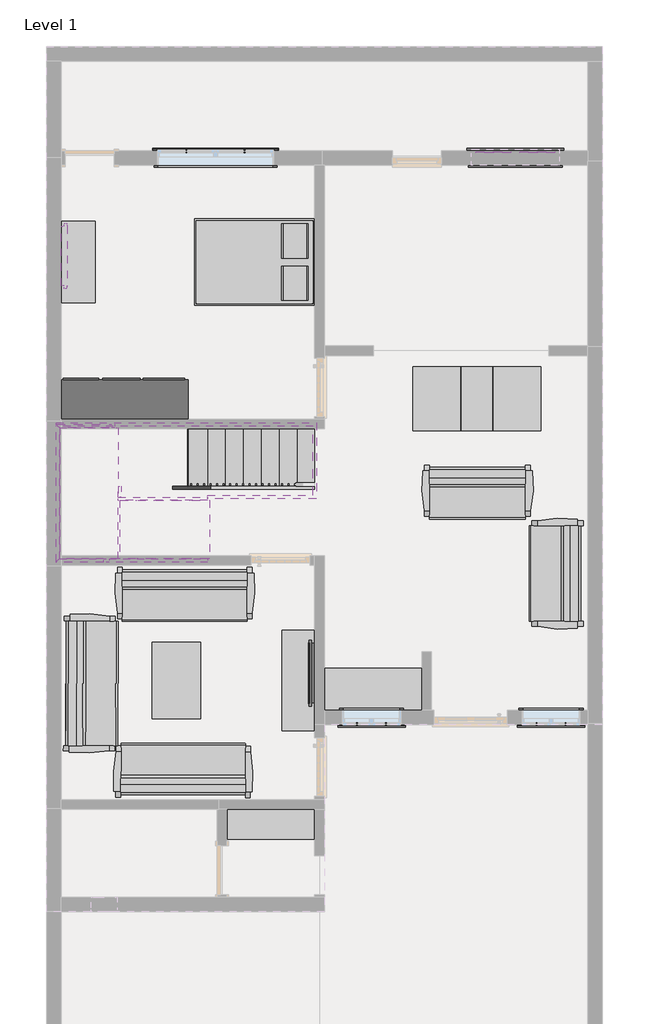
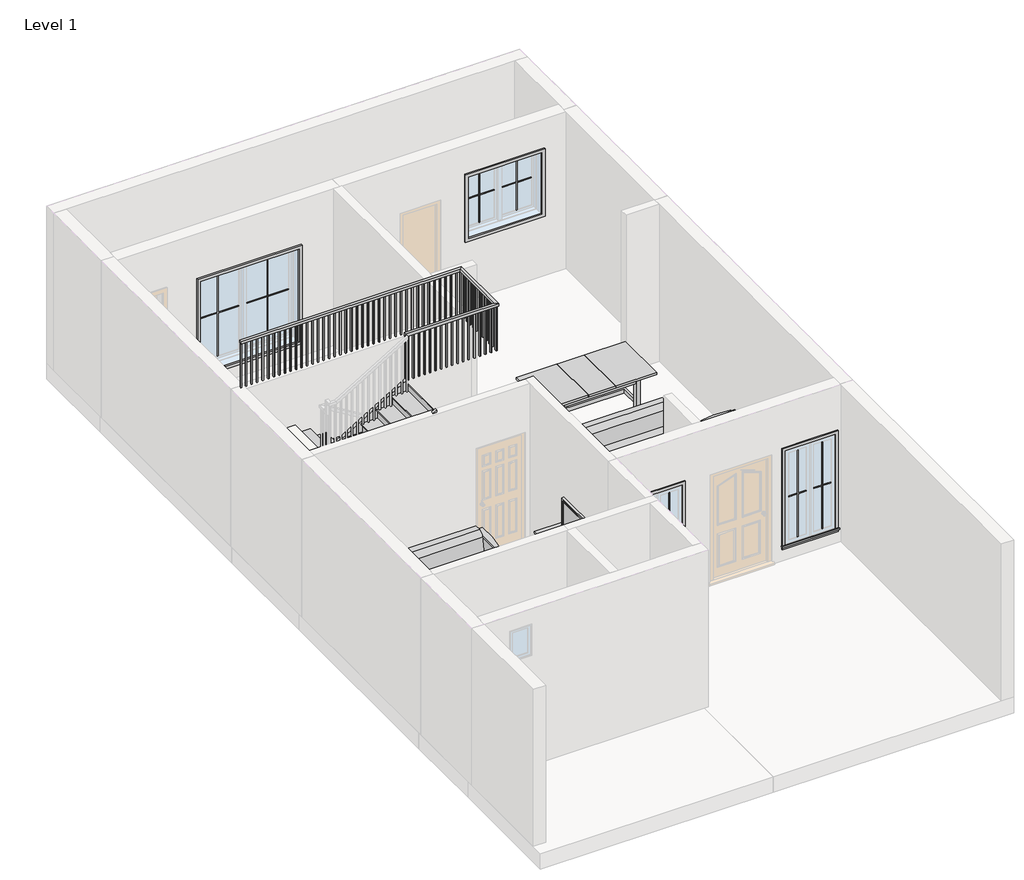
# One storey, part 3 of 3: 19 proxies, 12 furniture elements, 8 members, 2 stair flights, 1 railing, 1 slab.
"""IFC4 building model written with IfcOpenShell, lengths in millimetres."""

from ifc_helpers import new_model, si_unit, frame, origin, place, context, project, spatial, polyline, outline, extrude, faceted_brep, transform, mapped, element, save
from components import generic_models_374839be, muntin_pattern_2x2_muntin_pattern_2x2_0a037076, muntin_pattern_2x2_muntin_pattern_2x2_e6f69628, muntin_pattern_2x2_muntin_pattern_2x2_cdb221ef, muntin_pattern_2x2_muntin_pattern_2x2_811e8f4b, muntin_pattern_2x2_muntin_pattern_2x2_a158773a, muntin_pattern_2x2_muntin_pattern_2x2_9767bead, trim_window_exterior_flat_with_sill_b601e94a, trim_window_exterior_flat_with_sill_5276bcf3, trim_window_exterior_flat_with_sill_c2ca58d6, trim_window_interior_flat_picture_frame_bfefb25c, trim_window_interior_flat_picture_frame_3949a48f, trim_window_interior_flat_picture_frame_d9cdb79e, bath_1_bath_1_5f45cd17, room_1_room_1_fc48c56b, furniture_bed_1_1346x1880x355mm_double_93dec6ea, furniture_sideboard_1220x510x1070mm_0243b4aa, furniture_sideboard_1520x510x970mm_787d3fa7, furniture_sofa_2_1650mm_c7211d0d, furniture_sofa_2_2100x830x380mm_2cdf16e3, furniture_0b97a49d, furniture_table_coffee_glass_1200x760x330mm_bccf866f, furniture_table_dining_w_chairs_rectangular_2000x1000x750mm_b8cbee69, non_monolithic_landing_64c69633, stair_flight_cb879090, stair_flight_6d6c33ab

model = new_model("IFC4")

# Units and contexts
model_context = context("Model", 3, world=origin())
ifc_project = project(units=[si_unit("LENGTHUNIT", "METRE", prefix="MILLI")], contexts=[model_context])

# Site, building, storey
site = spatial("IfcSite", under=ifc_project)
building = spatial("IfcBuilding", under=site)
storey = spatial("IfcBuildingStorey", under=building, Name="Level 1", Elevation=0.0)

# Proxies
placement = place(None, origin())
generic_models_shape = generic_models_374839be(model_context)
element("IfcBuildingElementProxy", 1, Name="Generic Models", at=placement, inside=storey, context=model_context, shape_type="MappedRepresentation", body=[
    mapped(generic_models_shape, transform((0.0, 0.0, 0.0), x_axis=(1.0, 0.0, 0.0), y_axis=(0.0, 1.0, 0.0), z_axis=(0.0, 0.0, 1.0))),
])
muntin_pattern_2x2_muntin_pattern_2x2_shape = muntin_pattern_2x2_muntin_pattern_2x2_0a037076(model_context)
element("IfcBuildingElementProxy", 2, Name="Muntin Pattern_2x2 : Muntin Pattern_2x2", ObjectType="Muntin Pattern_2x2 : Muntin Pattern_2x2", at=placement, inside=storey, context=model_context, shape_type="MappedRepresentation", body=[
    mapped(muntin_pattern_2x2_muntin_pattern_2x2_shape, transform((-3390.5130972, 7136.1620892, 374.65), x_axis=(1.0, 0.0, 0.0), y_axis=(0.0, 1.0, 0.0), z_axis=(0.0, 0.0, 1.0))),
])
muntin_pattern_2x2_muntin_pattern_2x2_2_shape = muntin_pattern_2x2_muntin_pattern_2x2_e6f69628(model_context)
element("IfcBuildingElementProxy", 3, Name="Muntin Pattern_2x2 : Muntin Pattern_2x2", ObjectType="Muntin Pattern_2x2 : Muntin Pattern_2x2", at=placement, inside=storey, context=model_context, shape_type="MappedRepresentation", body=[
    mapped(muntin_pattern_2x2_muntin_pattern_2x2_2_shape, transform((-2479.2880972, 7136.1620892, 374.65), x_axis=(-1.0, 0.0, 0.0), y_axis=(0.0, -1.0, 0.0), z_axis=(0.0, 0.0, 1.0))),
])
muntin_pattern_2x2_muntin_pattern_2x2_3_shape = muntin_pattern_2x2_muntin_pattern_2x2_cdb221ef(model_context)
element("IfcBuildingElementProxy", 4, Name="Muntin Pattern_2x2 : Muntin Pattern_2x2", ObjectType="Muntin Pattern_2x2 : Muntin Pattern_2x2", at=placement, inside=storey, context=model_context, shape_type="MappedRepresentation", body=[
    mapped(muntin_pattern_2x2_muntin_pattern_2x2_3_shape, transform((1410.0869028, 7136.1620892, 1289.05), x_axis=(1.0, 0.0, 0.0), y_axis=(0.0, 1.0, 0.0), z_axis=(0.0, 0.0, 1.0))),
])
muntin_pattern_2x2_muntin_pattern_2x2_4_shape = muntin_pattern_2x2_muntin_pattern_2x2_811e8f4b(model_context)
element("IfcBuildingElementProxy", 5, Name="Muntin Pattern_2x2 : Muntin Pattern_2x2", ObjectType="Muntin Pattern_2x2 : Muntin Pattern_2x2", at=placement, inside=storey, context=model_context, shape_type="MappedRepresentation", body=[
    mapped(muntin_pattern_2x2_muntin_pattern_2x2_4_shape, transform((2092.7119028, 7136.1620892, 1289.05), x_axis=(-1.0, 0.0, 0.0), y_axis=(0.0, -1.0, 0.0), z_axis=(0.0, 0.0, 1.0))),
])
muntin_pattern_2x2_muntin_pattern_2x2_5_shape = muntin_pattern_2x2_muntin_pattern_2x2_a158773a(model_context)
element("IfcBuildingElementProxy", 6, Name="Muntin Pattern_2x2 : Muntin Pattern_2x2", ObjectType="Muntin Pattern_2x2 : Muntin Pattern_2x2", at=placement, inside=storey, context=model_context, shape_type="MappedRepresentation", body=[
    mapped(muntin_pattern_2x2_muntin_pattern_2x2_5_shape, transform((-269.4880972, -1810.9879108, 374.65), x_axis=(-1.0, 0.0, 0.0), y_axis=(0.0, -1.0, 0.0), z_axis=(0.0, 0.0, 1.0))),
])
element("IfcBuildingElementProxy", 7, Name="Muntin Pattern_2x2 : Muntin Pattern_2x2", ObjectType="Muntin Pattern_2x2 : Muntin Pattern_2x2", at=placement, inside=storey, context=model_context, shape_type="MappedRepresentation", body=[
    mapped(muntin_pattern_2x2_muntin_pattern_2x2_5_shape, transform((2537.2119028, -1810.9879108, 374.65), x_axis=(-1.0, 0.0, 0.0), y_axis=(0.0, -1.0, 0.0), z_axis=(0.0, 0.0, 1.0))),
])
muntin_pattern_2x2_muntin_pattern_2x2_6_shape = muntin_pattern_2x2_muntin_pattern_2x2_9767bead(model_context)
element("IfcBuildingElementProxy", 8, Name="Muntin Pattern_2x2 : Muntin Pattern_2x2", ObjectType="Muntin Pattern_2x2 : Muntin Pattern_2x2", at=placement, inside=storey, context=model_context, shape_type="MappedRepresentation", body=[
    mapped(muntin_pattern_2x2_muntin_pattern_2x2_6_shape, transform((-723.5130972, -1810.9879108, 374.65), x_axis=(1.0, 0.0, 0.0), y_axis=(0.0, 1.0, 0.0), z_axis=(0.0, 0.0, 1.0))),
])
element("IfcBuildingElementProxy", 9, Name="Muntin Pattern_2x2 : Muntin Pattern_2x2", ObjectType="Muntin Pattern_2x2 : Muntin Pattern_2x2", at=placement, inside=storey, context=model_context, shape_type="MappedRepresentation", body=[
    mapped(muntin_pattern_2x2_muntin_pattern_2x2_6_shape, transform((2083.1869028, -1810.9879108, 374.65), x_axis=(1.0, 0.0, 0.0), y_axis=(0.0, 1.0, 0.0), z_axis=(0.0, 0.0, 1.0))),
])
trim_window_exterior_flat_with_sill_shape = trim_window_exterior_flat_with_sill_b601e94a(model_context)
element("IfcBuildingElementProxy", 10, Name="Trim-Window-Exterior-Flat : with Sill", ObjectType="Trim-Window-Exterior-Flat : with Sill", at=placement, inside=storey, context=model_context, shape_type="MappedRepresentation", body=[
    mapped(trim_window_exterior_flat_with_sill_shape, transform((-2934.9005972, 7145.6870892, 2133.6), x_axis=(-1.0, 0.0, 0.0), y_axis=(0.0, 0.0, 1.0), z_axis=(0.0, 1.0, 0.0))),
])
trim_window_exterior_flat_with_sill_2_shape = trim_window_exterior_flat_with_sill_5276bcf3(model_context)
element("IfcBuildingElementProxy", 11, Name="Trim-Window-Exterior-Flat : with Sill", ObjectType="Trim-Window-Exterior-Flat : with Sill", at=placement, inside=storey, context=model_context, shape_type="MappedRepresentation", body=[
    mapped(trim_window_exterior_flat_with_sill_2_shape, transform((1751.3994028, 7145.6870892, 2438.4), x_axis=(-1.0, 0.0, 0.0), y_axis=(0.0, 0.0, 1.0), z_axis=(0.0, 1.0, 0.0))),
])
trim_window_exterior_flat_with_sill_3_shape = trim_window_exterior_flat_with_sill_c2ca58d6(model_context)
element("IfcBuildingElementProxy", 12, Name="Trim-Window-Exterior-Flat : with Sill", ObjectType="Trim-Window-Exterior-Flat : with Sill", at=placement, inside=storey, context=model_context, shape_type="MappedRepresentation", body=[
    mapped(trim_window_exterior_flat_with_sill_3_shape, transform((-496.5005972, -1820.5129108, 2133.6), x_axis=(1.0, 0.0, 0.0), y_axis=(0.0, 0.0, 1.0), z_axis=(0.0, -1.0, 0.0))),
])
element("IfcBuildingElementProxy", 13, Name="Trim-Window-Exterior-Flat : with Sill", ObjectType="Trim-Window-Exterior-Flat : with Sill", at=placement, inside=storey, context=model_context, shape_type="MappedRepresentation", body=[
    mapped(trim_window_exterior_flat_with_sill_3_shape, transform((2310.1994028, -1820.5129108, 2133.6), x_axis=(1.0, 0.0, 0.0), y_axis=(0.0, 0.0, 1.0), z_axis=(0.0, -1.0, 0.0))),
])
trim_window_interior_flat_picture_frame_shape = trim_window_interior_flat_picture_frame_bfefb25c(model_context)
element("IfcBuildingElementProxy", 14, Name="Trim-Window-Interior-Flat : Picture Frame", ObjectType="Trim-Window-Interior-Flat : Picture Frame", at=placement, inside=storey, context=model_context, shape_type="MappedRepresentation", body=[
    mapped(trim_window_interior_flat_picture_frame_shape, transform((-2934.9005972, 6917.0870892, 2133.6), x_axis=(1.0, 0.0, 0.0), y_axis=(0.0, 0.0, 1.0), z_axis=(0.0, -1.0, 0.0))),
])
trim_window_interior_flat_picture_frame_2_shape = trim_window_interior_flat_picture_frame_3949a48f(model_context)
element("IfcBuildingElementProxy", 15, Name="Trim-Window-Interior-Flat : Picture Frame", ObjectType="Trim-Window-Interior-Flat : Picture Frame", at=placement, inside=storey, context=model_context, shape_type="MappedRepresentation", body=[
    mapped(trim_window_interior_flat_picture_frame_2_shape, transform((1751.3994028, 6917.0870892, 2438.4), x_axis=(1.0, 0.0, 0.0), y_axis=(0.0, 0.0, 1.0), z_axis=(0.0, -1.0, 0.0))),
])
trim_window_interior_flat_picture_frame_3_shape = trim_window_interior_flat_picture_frame_d9cdb79e(model_context)
element("IfcBuildingElementProxy", 16, Name="Trim-Window-Interior-Flat : Picture Frame", ObjectType="Trim-Window-Interior-Flat : Picture Frame", at=placement, inside=storey, context=model_context, shape_type="MappedRepresentation", body=[
    mapped(trim_window_interior_flat_picture_frame_3_shape, transform((-496.5005972, -1591.9129108, 2133.6), x_axis=(-1.0, 0.0, 0.0), y_axis=(0.0, 0.0, 1.0), z_axis=(0.0, 1.0, 0.0))),
])
element("IfcBuildingElementProxy", 17, Name="Trim-Window-Interior-Flat : Picture Frame", ObjectType="Trim-Window-Interior-Flat : Picture Frame", at=placement, inside=storey, context=model_context, shape_type="MappedRepresentation", body=[
    mapped(trim_window_interior_flat_picture_frame_3_shape, transform((2310.1994028, -1591.9129108, 2133.6), x_axis=(-1.0, 0.0, 0.0), y_axis=(0.0, 0.0, 1.0), z_axis=(0.0, 1.0, 0.0))),
])
bath_1_bath_1_shape = bath_1_bath_1_5f45cd17(model_context)
element("IfcBuildingElementProxy", 18, Name="bath 1 : bath 1", ObjectType="bath 1 : bath 1", at=placement, inside=storey, context=model_context, shape_type="MappedRepresentation", body=[
    mapped(bath_1_bath_1_shape, transform((0.0, 0.0, 0.0), x_axis=(1.0, 0.0, 0.0), y_axis=(0.0, 1.0, 0.0), z_axis=(0.0, 0.0, 1.0))),
])
room_1_room_1_shape = room_1_room_1_fc48c56b(model_context)
element("IfcBuildingElementProxy", 19, Name="room 1 : room 1", ObjectType="room 1 : room 1", at=placement, inside=storey, context=model_context, shape_type="MappedRepresentation", body=[
    mapped(room_1_room_1_shape, transform((0.0, 0.0, 0.0), x_axis=(1.0, 0.0, 0.0), y_axis=(0.0, 1.0, 0.0), z_axis=(0.0, 0.0, 1.0))),
])

# Furniture
furniture_bed_1_1346x1880x355mm_double_shape = furniture_bed_1_1346x1880x355mm_double_93dec6ea(model_context)
element("IfcFurniture", 20, ObjectType="Furniture_Bed_1 : 1346x1880x355mm-Double", at=placement, inside=storey, context=model_context, shape_type="MappedRepresentation", body=[
    mapped(furniture_bed_1_1346x1880x355mm_double_shape, transform((-2091.071089, 5744.8395482, 0.0), x_axis=(0.0, -1.0, 0.0), y_axis=(1.0, 0.0, 0.0), z_axis=(0.0, 0.0, 1.0))),
])
furniture_sideboard_1220x510x1070mm_shape = furniture_sideboard_1220x510x1070mm_0243b4aa(model_context)
element("IfcFurniture", 21, ObjectType="Furniture_Sideboard : 1220x510x1070mm", at=placement, inside=storey, context=model_context, shape_type="MappedRepresentation", body=[
    mapped(furniture_sideboard_1220x510x1070mm_shape, transform((-5458.0635513, 5700.280349, 0.0), x_axis=(0.0, 1.0, 0.0), y_axis=(-1.0, 0.0, 0.0), z_axis=(0.0, 0.0, 1.0))),
])
furniture_sideboard_1520x510x970mm_shape = furniture_sideboard_1520x510x970mm_787d3fa7(model_context)
element("IfcFurniture", 22, ObjectType="Furniture_Sideboard : 1520x510x970mm", at=placement, inside=storey, context=model_context, shape_type="MappedRepresentation", body=[
    mapped(furniture_sideboard_1520x510x970mm_shape, transform((-2003.6635513, -836.9734915, 0.0), x_axis=(0.0, 1.0, 0.0), y_axis=(-1.0, 0.0, 0.0), z_axis=(0.0, 0.0, 1.0))),
])
furniture_sofa_2_1650mm_shape = furniture_sofa_2_1650mm_c7211d0d(model_context)
element("IfcFurniture", 23, ObjectType="Furniture_Sofa_2 : 1650mm", at=placement, inside=storey, context=model_context, shape_type="MappedRepresentation", body=[
    mapped(furniture_sofa_2_1650mm_shape, transform((2109.2895667, 820.2933392, 0.0), x_axis=(0.0, -1.0, 0.0), y_axis=(1.0, 0.0, 0.0), z_axis=(0.0, 0.0, 1.0))),
])
element("IfcFurniture", 24, ObjectType="Furniture_Sofa_2 : 1650mm", at=placement, inside=storey, context=model_context, shape_type="MappedRepresentation", body=[
    mapped(furniture_sofa_2_1650mm_shape, transform((880.1212465, 1534.5772531, 0.0), x_axis=(1.0, 0.0, 0.0), y_axis=(0.0, 1.0, 0.0), z_axis=(0.0, 0.0, 1.0))),
])
furniture_sofa_2_2100x830x380mm_shape = furniture_sofa_2_2100x830x380mm_2cdf16e3(model_context)
element("IfcFurniture", 25, ObjectType="Furniture_Sofa_2 : 2100x830x380mm", at=placement, inside=storey, context=model_context, shape_type="MappedRepresentation", body=[
    mapped(furniture_sofa_2_2100x830x380mm_shape, transform((-4606.7733815, -1454.7297414, 0.0), x_axis=(0.004438895051769032, 0.9999901480568293, 0.0), y_axis=(-0.9999901480568293, 0.004438895051769032, 0.0), z_axis=(0.0, 0.0, 1.0))),
])
element("IfcFurniture", 26, ObjectType="Furniture_Sofa_2 : 2100x830x380mm", at=placement, inside=storey, context=model_context, shape_type="MappedRepresentation", body=[
    mapped(furniture_sofa_2_2100x830x380mm_shape, transform((-3161.0077895, -2253.3666662, 0.0), x_axis=(-0.9999901480568293, 0.004438895051769032, 0.0), y_axis=(-0.004438895051769032, -0.9999901480568293, 0.0), z_axis=(0.0, 0.0, 1.0))),
])
element("IfcFurniture", 27, ObjectType="Furniture_Sofa_2 : 2100x830x380mm", at=placement, inside=storey, context=model_context, shape_type="MappedRepresentation", body=[
    mapped(furniture_sofa_2_2100x830x380mm_shape, transform((-3696.1068472, -65.6227469, 0.0), x_axis=(1.0, 0.0, 0.0), y_axis=(0.0, 1.0, 0.0), z_axis=(0.0, 0.0, 1.0))),
])
furniture_shape = furniture_0b97a49d(model_context)
element("IfcFurniture", 28, ObjectType="Furniture_TV_Plasma : 42\"", at=placement, inside=storey, context=model_context, shape_type="MappedRepresentation", body=[
    mapped(furniture_shape, transform((-1385.5005972, -956.9129108, 914.4), x_axis=(0.0, -1.0, 0.0), y_axis=(1.0, 0.0, 0.0), z_axis=(0.0, 0.0, 1.0))),
])
element("IfcFurniture", 29, ObjectType="Furniture_TV_Plasma : 42\"", at=placement, inside=storey, context=model_context, shape_type="MappedRepresentation", body=[
    mapped(furniture_shape, transform((-5347.9005972, 5444.1870892, 1219.2), x_axis=(0.0, 1.0, 0.0), y_axis=(-1.0, 0.0, 0.0), z_axis=(0.0, 0.0, 1.0))),
])
furniture_table_coffee_glass_1200x760x330mm_shape = furniture_table_coffee_glass_1200x760x330mm_bccf866f(model_context)
element("IfcFurniture", 30, ObjectType="Furniture_Table_Coffee_Glass : 1200x760x330mm", at=placement, inside=storey, context=model_context, shape_type="MappedRepresentation", body=[
    mapped(furniture_table_coffee_glass_1200x760x330mm_shape, transform((-3180.2784522, -1733.8037647, 0.0), x_axis=(0.0, 1.0, 0.0), y_axis=(-1.0, 0.0, 0.0), z_axis=(0.0, 0.0, 1.0))),
])
furniture_table_dining_w_chairs_rectangular_2000x1000x750mm_shape = furniture_table_dining_w_chairs_rectangular_2000x1000x750mm_b8cbee69(model_context)
element("IfcFurniture", 31, ObjectType="Furniture_Table_Dining_w-Chairs_Rectangular : 2000x1000x750mm_w-4_Seats", at=placement, inside=storey, context=model_context, shape_type="MappedRepresentation", body=[
    mapped(furniture_table_dining_w_chairs_rectangular_2000x1000x750mm_shape, transform((1034.1657547, 3225.7786522, 0.0), x_axis=(1.0, 0.0, 0.0), y_axis=(0.0, 1.0, 0.0), z_axis=(0.0, 0.0, 1.0))),
])

# Members
element("IfcMember", 32, ObjectType="Stringer - 2\" Width", at=placement, inside=storey, context=model_context, shape_type="SweptSolid", body=[
    extrude(outline(polyline([(0.0, -1385.5005972), (212.114512, -1385.5005972), (2043.9932998, -4408.1005972), (1687.5845383, -4408.1005972), (0.0, -1623.586109), (0.0, -1385.5005972)])), frame((0.0, 1854.295038, 0.0), z_axis=(0.0, 1.0, 0.0), x_axis=(0.0, 0.0, 1.0)), (0.0, 0.0, 1.0), 50.8),
])
element("IfcMember", 33, ObjectType="Stringer - 2\" Width", at=placement, inside=storey, context=model_context, shape_type="SweptSolid", body=[
    extrude(outline(polyline([(0.0, -1385.5005972), (212.114512, -1385.5005972), (2108.2, -4514.0416525), (1803.4, -4599.196109), (0.0, -1623.586109), (0.0, -1385.5005972)])), frame((0.0, 2819.495038, 0.0), z_axis=(0.0, 1.0, 0.0), x_axis=(0.0, 0.0, 1.0)), (0.0, 0.0, 1.0), 50.8),
])
element("IfcMember", 34, ObjectType="Stringer - 2\" Width", at=placement, inside=storey, context=model_context, shape_type="SweptSolid", body=[
    extrude(outline(polyline([(2244.114512, -4458.9005972), (1887.7057504, -4458.9005972), (2734.3724171, -3061.9005972), (3090.7811786, -3061.9005972), (2244.114512, -4458.9005972)])), frame((0.0, 1684.6870892, 0.0), z_axis=(0.0, 1.0, 0.0), x_axis=(0.0, 0.0, 1.0)), (0.0, 0.0, 1.0), 50.8),
])
element("IfcMember", 35, ObjectType="Stringer - 2\" Width", at=placement, inside=storey, context=model_context, shape_type="SweptSolid", body=[
    extrude(outline(polyline([(2108.2, -4683.1595419), (1803.4, -4598.0050854), (2734.3724171, -3061.9005972), (3090.7811786, -3061.9005972), (2108.2, -4683.1595419)])), frame((0.0, 719.4870892, 0.0), z_axis=(0.0, 1.0, 0.0), x_axis=(0.0, 0.0, 1.0)), (0.0, 0.0, 1.0), 50.8),
])
element("IfcMember", 36, ObjectType="Stringer - 2\" Width", at=placement, inside=storey, context=model_context, shape_type="SweptSolid", body=[
    extrude(outline(polyline([(-4408.1005972, 1735.4870892), (-4458.9005972, 1735.4870892), (-4458.9005972, 1905.095038), (-4408.1005972, 1905.095038), (-4408.1005972, 1735.4870892)])), frame((0.0, 0.0, 1803.4), z_axis=(0.0, 0.0, 1.0), x_axis=(1.0, 0.0, 0.0)), (0.0, 0.0, 1.0), 304.8),
])
element("IfcMember", 37, ObjectType="Stringer - 2\" Width", at=placement, inside=storey, context=model_context, shape_type="Brep", body=[
    faceted_brep([(-4514.0416525, 2819.495038, 2108.2), (-4514.0416525, 2870.295038, 2108.2), (-5424.1005972, 2870.295038, 2108.2), (-5373.3005972, 2819.495038, 2108.2), (-4599.196109, 2819.495038, 1803.4), (-5373.3005972, 2819.495038, 1803.4), (-4599.196109, 2870.295038, 1803.4), (-5424.1005972, 2870.295038, 1803.4)], [[[0, 1, 2, 3]], [[4, 0, 3, 5]], [[6, 4, 5, 7]], [[1, 6, 7, 2]], [[1, 0, 4, 6]], [[2, 7, 5, 3]]]),
])
element("IfcMember", 38, ObjectType="Stringer - 2\" Width", at=placement, inside=storey, context=model_context, shape_type="SweptSolid", body=[
    extrude(outline(polyline([(-5424.1005972, 2870.295038), (-5373.3005972, 2819.495038), (-5373.3005972, 770.2870892), (-5424.1005972, 719.4870892), (-5424.1005972, 2870.295038)])), frame((0.0, 0.0, 1803.4), z_axis=(0.0, 0.0, 1.0), x_axis=(1.0, 0.0, 0.0)), (0.0, 0.0, 1.0), 304.8),
])
element("IfcMember", 39, ObjectType="Stringer - 2\" Width", at=placement, inside=storey, context=model_context, shape_type="Brep", body=[
    faceted_brep([(-5373.3005972, 770.2870892, 2108.2), (-5424.1005972, 719.4870892, 2108.2), (-4683.1595419, 719.4870892, 2108.2), (-4683.1595419, 770.2870892, 2108.2), (-5373.3005972, 770.2870892, 1803.4), (-4598.0050854, 770.2870892, 1803.4), (-5424.1005972, 719.4870892, 1803.4), (-4598.0050854, 719.4870892, 1803.4)], [[[0, 1, 2, 3]], [[4, 0, 3, 5]], [[6, 4, 5, 7]], [[1, 6, 7, 2]], [[1, 0, 4, 6]], [[2, 7, 5, 3]]]),
])

# Railing
element("IfcRailing", 40, ObjectType="Handrail - Rectangular", at=placement, inside=storey, context=model_context, shape_type="SolidModel", body=[
    faceted_brep([(-5424.1005972, 2895.695038, 3962.4), (-5424.1005972, 2895.695038, 3911.6), (-5424.1005972, 2844.895038, 3911.6), (-5424.1005972, 2844.895038, 3962.4), (-1410.9005972, 2844.895038, 3911.6), (-1410.9005972, 2844.895038, 3962.4), (-1360.1005972, 2895.695038, 3962.4), (-1410.9005972, 1760.8870892, 3911.6), (-1410.9005972, 1760.8870892, 3962.4), (-1360.1005972, 1710.0870892, 3962.4), (-3061.9005972, 1710.0870892, 3962.4), (-3061.9005972, 1760.8870892, 3962.4), (-3061.9005972, 1760.8870892, 3911.6), (-3061.9005972, 1710.0870892, 3911.6), (-1360.1005972, 2895.695038, 3911.6), (-1360.1005972, 1710.0870892, 3911.6)], [[[0, 1, 2, 3]], [[3, 2, 4, 5]], [[0, 3, 5, 6]], [[5, 4, 7, 8]], [[6, 5, 8, 9]], [[10, 11, 12, 13]], [[8, 7, 12, 11]], [[9, 8, 11, 10]], [[1, 0, 6, 14]], [[2, 1, 14, 4]], [[14, 6, 9, 15]], [[4, 14, 15, 7]], [[15, 9, 10, 13]], [[7, 15, 13, 12]]]),
    extrude(outline(polyline([(-3001.5755972, 1745.0120892), (-3001.5755972, 1725.9620892), (-3020.6255972, 1725.9620892), (-3020.6255972, 1745.0120892), (-3001.5755972, 1745.0120892)])), frame((0.0, 0.0, 3048.0), z_axis=(0.0, 0.0, 1.0), x_axis=(1.0, 0.0, 0.0)), (0.0, 0.0, 1.0), 863.6),
    extrude(outline(polyline([(-2899.9755972, 1745.0120892), (-2899.9755972, 1725.9620892), (-2919.0255972, 1725.9620892), (-2919.0255972, 1745.0120892), (-2899.9755972, 1745.0120892)])), frame((0.0, 0.0, 3048.0), z_axis=(0.0, 0.0, 1.0), x_axis=(1.0, 0.0, 0.0)), (0.0, 0.0, 1.0), 863.6),
    extrude(outline(polyline([(-2798.3755972, 1745.0120892), (-2798.3755972, 1725.9620892), (-2817.4255972, 1725.9620892), (-2817.4255972, 1745.0120892), (-2798.3755972, 1745.0120892)])), frame((0.0, 0.0, 3048.0), z_axis=(0.0, 0.0, 1.0), x_axis=(1.0, 0.0, 0.0)), (0.0, 0.0, 1.0), 863.6),
    extrude(outline(polyline([(-2696.7755972, 1745.0120892), (-2696.7755972, 1725.9620892), (-2715.8255972, 1725.9620892), (-2715.8255972, 1745.0120892), (-2696.7755972, 1745.0120892)])), frame((0.0, 0.0, 3048.0), z_axis=(0.0, 0.0, 1.0), x_axis=(1.0, 0.0, 0.0)), (0.0, 0.0, 1.0), 863.6),
    extrude(outline(polyline([(-2595.1755972, 1745.0120892), (-2595.1755972, 1725.9620892), (-2614.2255972, 1725.9620892), (-2614.2255972, 1745.0120892), (-2595.1755972, 1745.0120892)])), frame((0.0, 0.0, 3048.0), z_axis=(0.0, 0.0, 1.0), x_axis=(1.0, 0.0, 0.0)), (0.0, 0.0, 1.0), 863.6),
    extrude(outline(polyline([(-2493.5755972, 1745.0120892), (-2493.5755972, 1725.9620892), (-2512.6255972, 1725.9620892), (-2512.6255972, 1745.0120892), (-2493.5755972, 1745.0120892)])), frame((0.0, 0.0, 3048.0), z_axis=(0.0, 0.0, 1.0), x_axis=(1.0, 0.0, 0.0)), (0.0, 0.0, 1.0), 863.6),
    extrude(outline(polyline([(-2391.9755972, 1745.0120892), (-2391.9755972, 1725.9620892), (-2411.0255972, 1725.9620892), (-2411.0255972, 1745.0120892), (-2391.9755972, 1745.0120892)])), frame((0.0, 0.0, 3048.0), z_axis=(0.0, 0.0, 1.0), x_axis=(1.0, 0.0, 0.0)), (0.0, 0.0, 1.0), 863.6),
    extrude(outline(polyline([(-2290.3755972, 1745.0120892), (-2290.3755972, 1725.9620892), (-2309.4255972, 1725.9620892), (-2309.4255972, 1745.0120892), (-2290.3755972, 1745.0120892)])), frame((0.0, 0.0, 3048.0), z_axis=(0.0, 0.0, 1.0), x_axis=(1.0, 0.0, 0.0)), (0.0, 0.0, 1.0), 863.6),
    extrude(outline(polyline([(-2188.7755972, 1745.0120892), (-2188.7755972, 1725.9620892), (-2207.8255972, 1725.9620892), (-2207.8255972, 1745.0120892), (-2188.7755972, 1745.0120892)])), frame((0.0, 0.0, 3048.0), z_axis=(0.0, 0.0, 1.0), x_axis=(1.0, 0.0, 0.0)), (0.0, 0.0, 1.0), 863.6),
    extrude(outline(polyline([(-2087.1755972, 1745.0120892), (-2087.1755972, 1725.9620892), (-2106.2255972, 1725.9620892), (-2106.2255972, 1745.0120892), (-2087.1755972, 1745.0120892)])), frame((0.0, 0.0, 3048.0), z_axis=(0.0, 0.0, 1.0), x_axis=(1.0, 0.0, 0.0)), (0.0, 0.0, 1.0), 863.6),
    extrude(outline(polyline([(-1985.5755972, 1745.0120892), (-1985.5755972, 1725.9620892), (-2004.6255972, 1725.9620892), (-2004.6255972, 1745.0120892), (-1985.5755972, 1745.0120892)])), frame((0.0, 0.0, 3048.0), z_axis=(0.0, 0.0, 1.0), x_axis=(1.0, 0.0, 0.0)), (0.0, 0.0, 1.0), 863.6),
    extrude(outline(polyline([(-1883.9755972, 1745.0120892), (-1883.9755972, 1725.9620892), (-1903.0255972, 1725.9620892), (-1903.0255972, 1745.0120892), (-1883.9755972, 1745.0120892)])), frame((0.0, 0.0, 3048.0), z_axis=(0.0, 0.0, 1.0), x_axis=(1.0, 0.0, 0.0)), (0.0, 0.0, 1.0), 863.6),
    extrude(outline(polyline([(-1782.3755972, 1745.0120892), (-1782.3755972, 1725.9620892), (-1801.4255972, 1725.9620892), (-1801.4255972, 1745.0120892), (-1782.3755972, 1745.0120892)])), frame((0.0, 0.0, 3048.0), z_axis=(0.0, 0.0, 1.0), x_axis=(1.0, 0.0, 0.0)), (0.0, 0.0, 1.0), 863.6),
    extrude(outline(polyline([(-1680.7755972, 1745.0120892), (-1680.7755972, 1725.9620892), (-1699.8255972, 1725.9620892), (-1699.8255972, 1745.0120892), (-1680.7755972, 1745.0120892)])), frame((0.0, 0.0, 3048.0), z_axis=(0.0, 0.0, 1.0), x_axis=(1.0, 0.0, 0.0)), (0.0, 0.0, 1.0), 863.6),
    extrude(outline(polyline([(-1579.1755972, 1745.0120892), (-1579.1755972, 1725.9620892), (-1598.2255972, 1725.9620892), (-1598.2255972, 1745.0120892), (-1579.1755972, 1745.0120892)])), frame((0.0, 0.0, 3048.0), z_axis=(0.0, 0.0, 1.0), x_axis=(1.0, 0.0, 0.0)), (0.0, 0.0, 1.0), 863.6),
    extrude(outline(polyline([(-1477.5755972, 1745.0120892), (-1477.5755972, 1725.9620892), (-1496.6255972, 1725.9620892), (-1496.6255972, 1745.0120892), (-1477.5755972, 1745.0120892)])), frame((0.0, 0.0, 3048.0), z_axis=(0.0, 0.0, 1.0), x_axis=(1.0, 0.0, 0.0)), (0.0, 0.0, 1.0), 863.6),
    extrude(outline(polyline([(-1395.0255972, 1762.220038), (-1375.9755972, 1762.220038), (-1375.9755972, 1743.170038), (-1395.0255972, 1743.170038), (-1395.0255972, 1762.220038)])), frame((0.0, 0.0, 3048.0), z_axis=(0.0, 0.0, 1.0), x_axis=(1.0, 0.0, 0.0)), (0.0, 0.0, 1.0), 863.6),
    extrude(outline(polyline([(-1395.0255972, 1863.820038), (-1375.9755972, 1863.820038), (-1375.9755972, 1844.770038), (-1395.0255972, 1844.770038), (-1395.0255972, 1863.820038)])), frame((0.0, 0.0, 3048.0), z_axis=(0.0, 0.0, 1.0), x_axis=(1.0, 0.0, 0.0)), (0.0, 0.0, 1.0), 863.6),
    extrude(outline(polyline([(-1395.0255972, 1965.420038), (-1375.9755972, 1965.420038), (-1375.9755972, 1946.370038), (-1395.0255972, 1946.370038), (-1395.0255972, 1965.420038)])), frame((0.0, 0.0, 3048.0), z_axis=(0.0, 0.0, 1.0), x_axis=(1.0, 0.0, 0.0)), (0.0, 0.0, 1.0), 863.6),
    extrude(outline(polyline([(-1395.0255972, 2067.020038), (-1375.9755972, 2067.020038), (-1375.9755972, 2047.970038), (-1395.0255972, 2047.970038), (-1395.0255972, 2067.020038)])), frame((0.0, 0.0, 3048.0), z_axis=(0.0, 0.0, 1.0), x_axis=(1.0, 0.0, 0.0)), (0.0, 0.0, 1.0), 863.6),
    extrude(outline(polyline([(-1395.0255972, 2168.620038), (-1375.9755972, 2168.620038), (-1375.9755972, 2149.570038), (-1395.0255972, 2149.570038), (-1395.0255972, 2168.620038)])), frame((0.0, 0.0, 3048.0), z_axis=(0.0, 0.0, 1.0), x_axis=(1.0, 0.0, 0.0)), (0.0, 0.0, 1.0), 863.6),
    extrude(outline(polyline([(-1395.0255972, 2270.220038), (-1375.9755972, 2270.220038), (-1375.9755972, 2251.170038), (-1395.0255972, 2251.170038), (-1395.0255972, 2270.220038)])), frame((0.0, 0.0, 3048.0), z_axis=(0.0, 0.0, 1.0), x_axis=(1.0, 0.0, 0.0)), (0.0, 0.0, 1.0), 863.6),
    extrude(outline(polyline([(-1395.0255972, 2371.820038), (-1375.9755972, 2371.820038), (-1375.9755972, 2352.770038), (-1395.0255972, 2352.770038), (-1395.0255972, 2371.820038)])), frame((0.0, 0.0, 3048.0), z_axis=(0.0, 0.0, 1.0), x_axis=(1.0, 0.0, 0.0)), (0.0, 0.0, 1.0), 863.6),
    extrude(outline(polyline([(-1395.0255972, 2473.420038), (-1375.9755972, 2473.420038), (-1375.9755972, 2454.370038), (-1395.0255972, 2454.370038), (-1395.0255972, 2473.420038)])), frame((0.0, 0.0, 3048.0), z_axis=(0.0, 0.0, 1.0), x_axis=(1.0, 0.0, 0.0)), (0.0, 0.0, 1.0), 863.6),
    extrude(outline(polyline([(-1395.0255972, 2575.020038), (-1375.9755972, 2575.020038), (-1375.9755972, 2555.970038), (-1395.0255972, 2555.970038), (-1395.0255972, 2575.020038)])), frame((0.0, 0.0, 3048.0), z_axis=(0.0, 0.0, 1.0), x_axis=(1.0, 0.0, 0.0)), (0.0, 0.0, 1.0), 863.6),
    extrude(outline(polyline([(-1395.0255972, 2676.620038), (-1375.9755972, 2676.620038), (-1375.9755972, 2657.570038), (-1395.0255972, 2657.570038), (-1395.0255972, 2676.620038)])), frame((0.0, 0.0, 3048.0), z_axis=(0.0, 0.0, 1.0), x_axis=(1.0, 0.0, 0.0)), (0.0, 0.0, 1.0), 863.6),
    extrude(outline(polyline([(-1395.0255972, 2778.220038), (-1375.9755972, 2778.220038), (-1375.9755972, 2759.170038), (-1395.0255972, 2759.170038), (-1395.0255972, 2778.220038)])), frame((0.0, 0.0, 3048.0), z_axis=(0.0, 0.0, 1.0), x_axis=(1.0, 0.0, 0.0)), (0.0, 0.0, 1.0), 863.6),
    extrude(outline(polyline([(-1471.2255972, 2860.770038), (-1471.2255972, 2879.820038), (-1452.1755972, 2879.820038), (-1452.1755972, 2860.770038), (-1471.2255972, 2860.770038)])), frame((0.0, 0.0, 3048.0), z_axis=(0.0, 0.0, 1.0), x_axis=(1.0, 0.0, 0.0)), (0.0, 0.0, 1.0), 863.6),
    extrude(outline(polyline([(-1572.8255972, 2860.770038), (-1572.8255972, 2879.820038), (-1553.7755972, 2879.820038), (-1553.7755972, 2860.770038), (-1572.8255972, 2860.770038)])), frame((0.0, 0.0, 3048.0), z_axis=(0.0, 0.0, 1.0), x_axis=(1.0, 0.0, 0.0)), (0.0, 0.0, 1.0), 863.6),
    extrude(outline(polyline([(-1674.4255972, 2860.770038), (-1674.4255972, 2879.820038), (-1655.3755972, 2879.820038), (-1655.3755972, 2860.770038), (-1674.4255972, 2860.770038)])), frame((0.0, 0.0, 3048.0), z_axis=(0.0, 0.0, 1.0), x_axis=(1.0, 0.0, 0.0)), (0.0, 0.0, 1.0), 863.6),
    extrude(outline(polyline([(-1776.0255972, 2860.770038), (-1776.0255972, 2879.820038), (-1756.9755972, 2879.820038), (-1756.9755972, 2860.770038), (-1776.0255972, 2860.770038)])), frame((0.0, 0.0, 3048.0), z_axis=(0.0, 0.0, 1.0), x_axis=(1.0, 0.0, 0.0)), (0.0, 0.0, 1.0), 863.6),
    extrude(outline(polyline([(-1877.6255972, 2860.770038), (-1877.6255972, 2879.820038), (-1858.5755972, 2879.820038), (-1858.5755972, 2860.770038), (-1877.6255972, 2860.770038)])), frame((0.0, 0.0, 3048.0), z_axis=(0.0, 0.0, 1.0), x_axis=(1.0, 0.0, 0.0)), (0.0, 0.0, 1.0), 863.6),
    extrude(outline(polyline([(-1979.2255972, 2860.770038), (-1979.2255972, 2879.820038), (-1960.1755972, 2879.820038), (-1960.1755972, 2860.770038), (-1979.2255972, 2860.770038)])), frame((0.0, 0.0, 3048.0), z_axis=(0.0, 0.0, 1.0), x_axis=(1.0, 0.0, 0.0)), (0.0, 0.0, 1.0), 863.6),
    extrude(outline(polyline([(-2080.8255972, 2860.770038), (-2080.8255972, 2879.820038), (-2061.7755972, 2879.820038), (-2061.7755972, 2860.770038), (-2080.8255972, 2860.770038)])), frame((0.0, 0.0, 3048.0), z_axis=(0.0, 0.0, 1.0), x_axis=(1.0, 0.0, 0.0)), (0.0, 0.0, 1.0), 863.6),
    extrude(outline(polyline([(-2182.4255972, 2860.770038), (-2182.4255972, 2879.820038), (-2163.3755972, 2879.820038), (-2163.3755972, 2860.770038), (-2182.4255972, 2860.770038)])), frame((0.0, 0.0, 3048.0), z_axis=(0.0, 0.0, 1.0), x_axis=(1.0, 0.0, 0.0)), (0.0, 0.0, 1.0), 863.6),
    extrude(outline(polyline([(-2284.0255972, 2860.770038), (-2284.0255972, 2879.820038), (-2264.9755972, 2879.820038), (-2264.9755972, 2860.770038), (-2284.0255972, 2860.770038)])), frame((0.0, 0.0, 3048.0), z_axis=(0.0, 0.0, 1.0), x_axis=(1.0, 0.0, 0.0)), (0.0, 0.0, 1.0), 863.6),
    extrude(outline(polyline([(-2385.6255972, 2860.770038), (-2385.6255972, 2879.820038), (-2366.5755972, 2879.820038), (-2366.5755972, 2860.770038), (-2385.6255972, 2860.770038)])), frame((0.0, 0.0, 3048.0), z_axis=(0.0, 0.0, 1.0), x_axis=(1.0, 0.0, 0.0)), (0.0, 0.0, 1.0), 863.6),
    extrude(outline(polyline([(-2487.2255972, 2860.770038), (-2487.2255972, 2879.820038), (-2468.1755972, 2879.820038), (-2468.1755972, 2860.770038), (-2487.2255972, 2860.770038)])), frame((0.0, 0.0, 3048.0), z_axis=(0.0, 0.0, 1.0), x_axis=(1.0, 0.0, 0.0)), (0.0, 0.0, 1.0), 863.6),
    extrude(outline(polyline([(-2588.8255972, 2860.770038), (-2588.8255972, 2879.820038), (-2569.7755972, 2879.820038), (-2569.7755972, 2860.770038), (-2588.8255972, 2860.770038)])), frame((0.0, 0.0, 3048.0), z_axis=(0.0, 0.0, 1.0), x_axis=(1.0, 0.0, 0.0)), (0.0, 0.0, 1.0), 863.6),
    extrude(outline(polyline([(-2690.4255972, 2860.770038), (-2690.4255972, 2879.820038), (-2671.3755972, 2879.820038), (-2671.3755972, 2860.770038), (-2690.4255972, 2860.770038)])), frame((0.0, 0.0, 3048.0), z_axis=(0.0, 0.0, 1.0), x_axis=(1.0, 0.0, 0.0)), (0.0, 0.0, 1.0), 863.6),
    extrude(outline(polyline([(-2792.0255972, 2860.770038), (-2792.0255972, 2879.820038), (-2772.9755972, 2879.820038), (-2772.9755972, 2860.770038), (-2792.0255972, 2860.770038)])), frame((0.0, 0.0, 3048.0), z_axis=(0.0, 0.0, 1.0), x_axis=(1.0, 0.0, 0.0)), (0.0, 0.0, 1.0), 863.6),
    extrude(outline(polyline([(-2893.6255972, 2860.770038), (-2893.6255972, 2879.820038), (-2874.5755972, 2879.820038), (-2874.5755972, 2860.770038), (-2893.6255972, 2860.770038)])), frame((0.0, 0.0, 3048.0), z_axis=(0.0, 0.0, 1.0), x_axis=(1.0, 0.0, 0.0)), (0.0, 0.0, 1.0), 863.6),
    extrude(outline(polyline([(-2995.2255972, 2860.770038), (-2995.2255972, 2879.820038), (-2976.1755972, 2879.820038), (-2976.1755972, 2860.770038), (-2995.2255972, 2860.770038)])), frame((0.0, 0.0, 3048.0), z_axis=(0.0, 0.0, 1.0), x_axis=(1.0, 0.0, 0.0)), (0.0, 0.0, 1.0), 863.6),
    extrude(outline(polyline([(-3096.8255972, 2860.770038), (-3096.8255972, 2879.820038), (-3077.7755972, 2879.820038), (-3077.7755972, 2860.770038), (-3096.8255972, 2860.770038)])), frame((0.0, 0.0, 3048.0), z_axis=(0.0, 0.0, 1.0), x_axis=(1.0, 0.0, 0.0)), (0.0, 0.0, 1.0), 863.6),
    extrude(outline(polyline([(-3198.4255972, 2860.770038), (-3198.4255972, 2879.820038), (-3179.3755972, 2879.820038), (-3179.3755972, 2860.770038), (-3198.4255972, 2860.770038)])), frame((0.0, 0.0, 3048.0), z_axis=(0.0, 0.0, 1.0), x_axis=(1.0, 0.0, 0.0)), (0.0, 0.0, 1.0), 863.6),
    extrude(outline(polyline([(-3300.0255972, 2860.770038), (-3300.0255972, 2879.820038), (-3280.9755972, 2879.820038), (-3280.9755972, 2860.770038), (-3300.0255972, 2860.770038)])), frame((0.0, 0.0, 3048.0), z_axis=(0.0, 0.0, 1.0), x_axis=(1.0, 0.0, 0.0)), (0.0, 0.0, 1.0), 863.6),
    extrude(outline(polyline([(-3401.6255972, 2860.770038), (-3401.6255972, 2879.820038), (-3382.5755972, 2879.820038), (-3382.5755972, 2860.770038), (-3401.6255972, 2860.770038)])), frame((0.0, 0.0, 3048.0), z_axis=(0.0, 0.0, 1.0), x_axis=(1.0, 0.0, 0.0)), (0.0, 0.0, 1.0), 863.6),
    extrude(outline(polyline([(-3503.2255972, 2860.770038), (-3503.2255972, 2879.820038), (-3484.1755972, 2879.820038), (-3484.1755972, 2860.770038), (-3503.2255972, 2860.770038)])), frame((0.0, 0.0, 3048.0), z_axis=(0.0, 0.0, 1.0), x_axis=(1.0, 0.0, 0.0)), (0.0, 0.0, 1.0), 863.6),
    extrude(outline(polyline([(-3604.8255972, 2860.770038), (-3604.8255972, 2879.820038), (-3585.7755972, 2879.820038), (-3585.7755972, 2860.770038), (-3604.8255972, 2860.770038)])), frame((0.0, 0.0, 3048.0), z_axis=(0.0, 0.0, 1.0), x_axis=(1.0, 0.0, 0.0)), (0.0, 0.0, 1.0), 863.6),
    extrude(outline(polyline([(-3706.4255972, 2860.770038), (-3706.4255972, 2879.820038), (-3687.3755972, 2879.820038), (-3687.3755972, 2860.770038), (-3706.4255972, 2860.770038)])), frame((0.0, 0.0, 3048.0), z_axis=(0.0, 0.0, 1.0), x_axis=(1.0, 0.0, 0.0)), (0.0, 0.0, 1.0), 863.6),
    extrude(outline(polyline([(-3808.0255972, 2860.770038), (-3808.0255972, 2879.820038), (-3788.9755972, 2879.820038), (-3788.9755972, 2860.770038), (-3808.0255972, 2860.770038)])), frame((0.0, 0.0, 3048.0), z_axis=(0.0, 0.0, 1.0), x_axis=(1.0, 0.0, 0.0)), (0.0, 0.0, 1.0), 863.6),
    extrude(outline(polyline([(-3909.6255972, 2860.770038), (-3909.6255972, 2879.820038), (-3890.5755972, 2879.820038), (-3890.5755972, 2860.770038), (-3909.6255972, 2860.770038)])), frame((0.0, 0.0, 3048.0), z_axis=(0.0, 0.0, 1.0), x_axis=(1.0, 0.0, 0.0)), (0.0, 0.0, 1.0), 863.6),
    extrude(outline(polyline([(-4011.2255972, 2860.770038), (-4011.2255972, 2879.820038), (-3992.1755972, 2879.820038), (-3992.1755972, 2860.770038), (-4011.2255972, 2860.770038)])), frame((0.0, 0.0, 3048.0), z_axis=(0.0, 0.0, 1.0), x_axis=(1.0, 0.0, 0.0)), (0.0, 0.0, 1.0), 863.6),
    extrude(outline(polyline([(-4112.8255972, 2860.770038), (-4112.8255972, 2879.820038), (-4093.7755972, 2879.820038), (-4093.7755972, 2860.770038), (-4112.8255972, 2860.770038)])), frame((0.0, 0.0, 3048.0), z_axis=(0.0, 0.0, 1.0), x_axis=(1.0, 0.0, 0.0)), (0.0, 0.0, 1.0), 863.6),
    extrude(outline(polyline([(-4214.4255972, 2860.770038), (-4214.4255972, 2879.820038), (-4195.3755972, 2879.820038), (-4195.3755972, 2860.770038), (-4214.4255972, 2860.770038)])), frame((0.0, 0.0, 3048.0), z_axis=(0.0, 0.0, 1.0), x_axis=(1.0, 0.0, 0.0)), (0.0, 0.0, 1.0), 863.6),
    extrude(outline(polyline([(-4316.0255972, 2860.770038), (-4316.0255972, 2879.820038), (-4296.9755972, 2879.820038), (-4296.9755972, 2860.770038), (-4316.0255972, 2860.770038)])), frame((0.0, 0.0, 3048.0), z_axis=(0.0, 0.0, 1.0), x_axis=(1.0, 0.0, 0.0)), (0.0, 0.0, 1.0), 863.6),
    extrude(outline(polyline([(-4417.6255972, 2860.770038), (-4417.6255972, 2879.820038), (-4398.5755972, 2879.820038), (-4398.5755972, 2860.770038), (-4417.6255972, 2860.770038)])), frame((0.0, 0.0, 3048.0), z_axis=(0.0, 0.0, 1.0), x_axis=(1.0, 0.0, 0.0)), (0.0, 0.0, 1.0), 863.6),
    extrude(outline(polyline([(-4519.2255972, 2860.770038), (-4519.2255972, 2879.820038), (-4500.1755972, 2879.820038), (-4500.1755972, 2860.770038), (-4519.2255972, 2860.770038)])), frame((0.0, 0.0, 3048.0), z_axis=(0.0, 0.0, 1.0), x_axis=(1.0, 0.0, 0.0)), (0.0, 0.0, 1.0), 863.6),
    extrude(outline(polyline([(-4620.8255972, 2860.770038), (-4620.8255972, 2879.820038), (-4601.7755972, 2879.820038), (-4601.7755972, 2860.770038), (-4620.8255972, 2860.770038)])), frame((0.0, 0.0, 3048.0), z_axis=(0.0, 0.0, 1.0), x_axis=(1.0, 0.0, 0.0)), (0.0, 0.0, 1.0), 863.6),
    extrude(outline(polyline([(-4722.4255972, 2860.770038), (-4722.4255972, 2879.820038), (-4703.3755972, 2879.820038), (-4703.3755972, 2860.770038), (-4722.4255972, 2860.770038)])), frame((0.0, 0.0, 3048.0), z_axis=(0.0, 0.0, 1.0), x_axis=(1.0, 0.0, 0.0)), (0.0, 0.0, 1.0), 863.6),
    extrude(outline(polyline([(-4824.0255972, 2860.770038), (-4824.0255972, 2879.820038), (-4804.9755972, 2879.820038), (-4804.9755972, 2860.770038), (-4824.0255972, 2860.770038)])), frame((0.0, 0.0, 3048.0), z_axis=(0.0, 0.0, 1.0), x_axis=(1.0, 0.0, 0.0)), (0.0, 0.0, 1.0), 863.6),
    extrude(outline(polyline([(-4925.6255972, 2860.770038), (-4925.6255972, 2879.820038), (-4906.5755972, 2879.820038), (-4906.5755972, 2860.770038), (-4925.6255972, 2860.770038)])), frame((0.0, 0.0, 3048.0), z_axis=(0.0, 0.0, 1.0), x_axis=(1.0, 0.0, 0.0)), (0.0, 0.0, 1.0), 863.6),
    extrude(outline(polyline([(-5027.2255972, 2860.770038), (-5027.2255972, 2879.820038), (-5008.1755972, 2879.820038), (-5008.1755972, 2860.770038), (-5027.2255972, 2860.770038)])), frame((0.0, 0.0, 3048.0), z_axis=(0.0, 0.0, 1.0), x_axis=(1.0, 0.0, 0.0)), (0.0, 0.0, 1.0), 863.6),
    extrude(outline(polyline([(-5128.8255972, 2860.770038), (-5128.8255972, 2879.820038), (-5109.7755972, 2879.820038), (-5109.7755972, 2860.770038), (-5128.8255972, 2860.770038)])), frame((0.0, 0.0, 3048.0), z_axis=(0.0, 0.0, 1.0), x_axis=(1.0, 0.0, 0.0)), (0.0, 0.0, 1.0), 863.6),
    extrude(outline(polyline([(-5230.4255972, 2860.770038), (-5230.4255972, 2879.820038), (-5211.3755972, 2879.820038), (-5211.3755972, 2860.770038), (-5230.4255972, 2860.770038)])), frame((0.0, 0.0, 3048.0), z_axis=(0.0, 0.0, 1.0), x_axis=(1.0, 0.0, 0.0)), (0.0, 0.0, 1.0), 863.6),
    extrude(outline(polyline([(-5332.0255972, 2860.770038), (-5332.0255972, 2879.820038), (-5312.9755972, 2879.820038), (-5312.9755972, 2860.770038), (-5332.0255972, 2860.770038)])), frame((0.0, 0.0, 3048.0), z_axis=(0.0, 0.0, 1.0), x_axis=(1.0, 0.0, 0.0)), (0.0, 0.0, 1.0), 863.6),
    extrude(outline(polyline([(-1395.0255972, 1745.0120892), (-1375.9755972, 1745.0120892), (-1375.9755972, 1725.9620892), (-1395.0255972, 1725.9620892), (-1395.0255972, 1745.0120892)])), frame((0.0, 0.0, 3048.0), z_axis=(0.0, 0.0, 1.0), x_axis=(1.0, 0.0, 0.0)), (0.0, 0.0, 1.0), 863.6),
    extrude(outline(polyline([(-1395.0255972, 2860.770038), (-1395.0255972, 2879.820038), (-1375.9755972, 2879.820038), (-1375.9755972, 2860.770038), (-1395.0255972, 2860.770038)])), frame((0.0, 0.0, 3048.0), z_axis=(0.0, 0.0, 1.0), x_axis=(1.0, 0.0, 0.0)), (0.0, 0.0, 1.0), 863.6),
    extrude(outline(polyline([(-3042.8505972, 1745.0120892), (-3042.8505972, 1725.9620892), (-3061.9005972, 1725.9620892), (-3061.9005972, 1745.0120892), (-3042.8505972, 1745.0120892)])), frame((0.0, 0.0, 3048.0), z_axis=(0.0, 0.0, 1.0), x_axis=(1.0, 0.0, 0.0)), (0.0, 0.0, 1.0), 863.6),
    extrude(outline(polyline([(-5424.1005972, 2860.770038), (-5424.1005972, 2879.820038), (-5405.0505972, 2879.820038), (-5405.0505972, 2860.770038), (-5424.1005972, 2860.770038)])), frame((0.0, 0.0, 3048.0), z_axis=(0.0, 0.0, 1.0), x_axis=(1.0, 0.0, 0.0)), (0.0, 0.0, 1.0), 863.6),
])

# Slab
non_monolithic_landing_shape = non_monolithic_landing_64c69633(model_context)
element("IfcSlab", 41, ObjectType="Non-Monolithic Landing", at=placement, inside=storey, context=model_context, shape_type="MappedRepresentation", body=[
    mapped(non_monolithic_landing_shape, transform((0.0, 0.0, 0.0), x_axis=(1.0, 0.0, 0.0), y_axis=(0.0, 1.0, 0.0), z_axis=(0.0, 0.0, 1.0))),
])

# Stair flights
stair_flight_shape = stair_flight_cb879090(model_context)
element("IfcStairFlight", 42, ObjectType="2\" Tread 1\" Nosing 1/4\" Riser", at=placement, inside=storey, context=model_context, shape_type="MappedRepresentation", body=[
    mapped(stair_flight_shape, transform((0.0, 0.0, 0.0), x_axis=(1.0, 0.0, 0.0), y_axis=(0.0, 1.0, 0.0), z_axis=(0.0, 0.0, 1.0))),
])
stair_flight_2_shape = stair_flight_6d6c33ab(model_context)
element("IfcStairFlight", 43, ObjectType="2\" Tread 1\" Nosing 1/4\" Riser", at=placement, inside=storey, context=model_context, shape_type="MappedRepresentation", body=[
    mapped(stair_flight_2_shape, transform((0.0, 0.0, 0.0), x_axis=(1.0, 0.0, 0.0), y_axis=(0.0, 1.0, 0.0), z_axis=(0.0, 0.0, 1.0))),
])

save(model, "model.ifc")

# Revit data of these elements
# Type "Muntin Pattern_2x2 : Muntin Pattern_2x2"
#   Width [instance default] = 4' - 0"
#   Thickness = 0' - 0 1/2"
#   Height [instance default] = 4' - 0"
#   Distance = 0' - 0 3/4"
#   Interior Material [instance default] = none
#   Exterior Material [instance default] = none
#   Default Elevation = 0
# Type "Trim-Window-Exterior-Flat : with Sill"
#   Trim Width = 0' - 2 1/4"
#   Trim Thickness_Picture Frame = 0' - 1 1/4"
#   Trim Thickness_with Sill = 0' - 0 3/4"
#   Sill Thickness = 0' - 1 1/4"
#   Opening Width [instance default] = 2' - 0"
#   Opening Height [instance default] = 3' - 0"
#   Default Elevation = 4' - 0"
#   Sill = yes
#   Picture Frame = no
#   Trim Material [instance default] = none
# Type "Trim-Window-Interior-Flat : Picture Frame"
#   Trim Thickness_Picture Frame = 0' - 1 1/4"
#   Trim Width = 0' - 2 1/4"
#   Trim Thickness_with Sill = 0' - 0 3/4"
#   Sill Thickness = 0' - 1 1/4"
#   Opening Width [instance default] = 2' - 0"
#   Opening Height [instance default] = 3' - 0"
#   Default Elevation = 4' - 0"
#   Sill = no
#   Picture Frame = yes
#   Trim Material [instance default] = none
# Type "Furniture_Bed_1 : 1346x1880x355mm-Double"
#   Keynote = "N"
#   Length = 6' - 2.01575"
#   Width = 4' - 4.99213"
#   Material Frame = Wood - Birch
#   Material Mattress = Textile - White
#   Default Elevation = 0
# Type "Furniture_Sideboard : 1220x510x1070mm"
#   Keynote = "N"
#   Depth = 1' - 8.07874"
#   Height = 3' - 5.33858"
#   Width = 4' - 0.0315"
#   Material = Wood - Cherry
#   Default Elevation = 0
#   Assembly Code = ""
# Type "Furniture_Sideboard : 1520x510x970mm"
#   Keynote = "N"
#   Depth = 1' - 8.07874"
#   Height = 3' - 2.18898"
#   Width = 4' - 11.84252"
#   Material = Wood - Cherry
#   Default Elevation = 0
#   Assembly Code = ""
# Type "Furniture_Sofa_2 : 1650mm"
#   Keynote = "N"
#   Length = 5' - 4.96063"
#   Material Sofa = Textile - Linen, Smooth
#   Material Frame = Metal - Chrome
#   Default Elevation = 0
# Type "Furniture_Sofa_2 : 2100x830x380mm"
#   Keynote = "N"
#   Length = 6' - 10.67717"
#   Material Sofa = Textile - Linen, Smooth
#   Material Frame = Metal - Chrome
#   Default Elevation = 0
# Type "Furniture_TV_Plasma : 42\""
#   Keynote = "N"
#   Assembly Code = "E2020200"
#   Depth = 0' - 3 1/2"
#   Height = 2' - 2"
#   Width = 3' - 4 1/2"
#   Material Cabinet = Plastic - Gray
#   Default Elevation = 0
# Type "Furniture_Table_Coffee_Glass : 1200x760x330mm"
#   Keynote = "N"
#   Height = 1' - 0.99213"
#   Length = 3' - 11.24409"
#   Width = 2' - 5.92126"
#   Material Base = Metal - Chrome
#   Material Top = Glass - Clear, Grey
#   Default Elevation = 0
#   Assembly Code = ""
# Type "Furniture_Table_Dining_w-Chairs_Rectangular : 2000x1000x750mm_w-4_Seats"
#   Keynote = "N"
#   Width = 3' - 3.37008"
#   Table Top Thickness = 0' - 1.5748"
#   Table Height = 2' - 5.52756"
#   Length = 6' - 6.74016"
#   Leg Width = 0' - 2.95276"
#   Leg Spacing Width = 2' - 7.49606"
#   Leg Spacing Length = 4' - 7.11811"
#   Chair Side Spacing = 2' - 3.55906"
#   Centre Piece = 1' - 7.68504"
#   Vis - End Chairs = no
#   Material Table = Wood - Birch
#   Material Chair Structure = Wood - Birch
#   Material Chair Covering = Fabric - Beige
#   Default Elevation = 0
# Type "Handrail - Rectangular"
#   Assembly Code = "C2010400"
#   built-in parameter 1008612 = 0.0416667 (stored number, unit not read)
#   built-in parameter 1008611 = 0.0416667 (stored number, unit not read)
#   built-in parameter 1008609 = 0.333333 (stored number, unit not read)
#   built-in parameter 1008604 = 0.166667 (stored number, unit not read)
#   built-in parameter 1008603 = 0.166667 (stored number, unit not read)
#   Railing Height = 3' - 0"
#   built-in parameter 1008630 = 2
#   built-in parameter 1008610 = 2
#   built-in parameter 1008618 = Baluster - Square : 3/4"
# Element 1 (IfcBuildingElementProxy)
#   Phase Created = New Construction
#   Materials on its faces: "Door - Panel"
# Elements 2, 3 (IfcBuildingElementProxy, "Muntin Pattern_2x2 : Muntin Pattern_2x2")
#   Width = 2' - 6 5/8"
#   Height = 5' - 6 1/2"
#   Interior Material = Wood - Stained
#   Exterior Material = Clad - White
#   Phase Created = New Construction
#   Materials on its faces: "Clad - White", "Wood - Stained"
# Elements 4, 5 (IfcBuildingElementProxy, "Muntin Pattern_2x2 : Muntin Pattern_2x2")
#   Width = 1' - 9 5/8"
#   Height = 3' - 6 1/2"
#   Interior Material = Wood - Stained
#   Exterior Material = Clad - White
#   Phase Created = New Construction
#   Materials on its faces: "Clad - White", "Wood - Stained"
# Elements 6, 7, 8, 9 (IfcBuildingElementProxy, "Muntin Pattern_2x2 : Muntin Pattern_2x2")
#   Width = 1' - 0 5/8"
#   Height = 5' - 6 1/2"
#   Interior Material = Wood - Stained
#   Exterior Material = Clad - White
#   Phase Created = New Construction
#   Materials on its faces: "Clad - White", "Wood - Stained"
# Element 10 (IfcBuildingElementProxy, "Trim-Window-Exterior-Flat : with Sill")
#   Opening Width = 6' - 0"
#   Opening Height = 6' - 0"
#   Trim Material = Clad - White
#   Phase Created = New Construction
#   Materials on its faces: "Clad - White"
# Element 11 (IfcBuildingElementProxy, "Trim-Window-Exterior-Flat : with Sill")
#   Opening Width = 4' - 6"
#   Opening Height = 4' - 0"
#   Trim Material = Clad - White
#   Phase Created = New Construction
#   Materials on its faces: "Clad - White"
# Elements 12, 13 (IfcBuildingElementProxy, "Trim-Window-Exterior-Flat : with Sill")
#   Opening Width = 3' - 0"
#   Opening Height = 6' - 0"
#   Trim Material = Clad - White
#   Phase Created = New Construction
#   Materials on its faces: "Clad - White"
# Element 14 (IfcBuildingElementProxy, "Trim-Window-Interior-Flat : Picture Frame")
#   Opening Width = 6' - 0"
#   Opening Height = 6' - 0"
#   Trim Material = Wood - Stained
#   Phase Created = New Construction
#   Materials on its faces: "Wood - Stained"
# Element 15 (IfcBuildingElementProxy, "Trim-Window-Interior-Flat : Picture Frame")
#   Opening Width = 4' - 6"
#   Opening Height = 4' - 0"
#   Trim Material = Wood - Stained
#   Phase Created = New Construction
#   Materials on its faces: "Wood - Stained"
# Elements 16, 17 (IfcBuildingElementProxy, "Trim-Window-Interior-Flat : Picture Frame")
#   Opening Width = 3' - 0"
#   Opening Height = 6' - 0"
#   Trim Material = Wood - Stained
#   Phase Created = New Construction
#   Materials on its faces: "Wood - Stained"
# Element 18 (IfcBuildingElementProxy, "bath 1 : bath 1")
#   Phase Created = New Construction
# Element 19 (IfcBuildingElementProxy, "room 1 : room 1")
#   Phase Created = New Construction
#   Materials on its faces: "Door - Frame/Mullion", "Door - Panel"
# Element 20 (IfcFurniture, "Furniture_Bed_1 : 1346x1880x355mm-Double")
#   Phase Created = New Construction
#   Materials on its faces: "Wood - Birch", "Textile - White"
# Element 21 (IfcFurniture, "Furniture_Sideboard : 1220x510x1070mm")
#   Phase Created = New Construction
#   Materials on its faces: "Wood - Cherry"
# Element 22 (IfcFurniture, "Furniture_Sideboard : 1520x510x970mm")
#   Phase Created = New Construction
#   Materials on its faces: "Wood - Cherry"
# Elements 23, 24 (IfcFurniture, "Furniture_Sofa_2 : 1650mm")
#   Phase Created = New Construction
#   Materials on its faces: "Textile - Linen, Smooth", "Metal - Chrome"
# Elements 25, 26, 27 (IfcFurniture, "Furniture_Sofa_2 : 2100x830x380mm")
#   Phase Created = New Construction
#   Materials on its faces: "Textile - Linen, Smooth", "Metal - Chrome"
# Elements 28, 29 (IfcFurniture, "Furniture_TV_Plasma : 42\"")
#   Phase Created = New Construction
#   Materials on its faces: "Plastic - Black", "Plastic - Gray", "Glass"
# Element 30 (IfcFurniture, "Furniture_Table_Coffee_Glass : 1200x760x330mm")
#   Phase Created = New Construction
#   Materials on its faces: "Metal - Chrome", "Glass - Clear, Grey"
# Element 31 (IfcFurniture, "Furniture_Table_Dining_w-Chairs_Rectangular : 2000x1000x750mm_w-4_Seats")
#   Phase Created = New Construction
#   Materials on its faces: "Wood - Birch"
# Elements 32, 33, 34, 35, 36, 37, 38, 39 (IfcMember, "Stringer - 2\" Width")
#   Phase Created = New Construction
# Element 40 (IfcRailing, "Handrail - Rectangular")
#   built-in parameter 1008621 = 10 (stored number, unit not read)
#   Phase Created = New Construction
# Element 41 (IfcSlab, "Non-Monolithic Landing")
#   Phase Created = New Construction
#   Materials on its faces: "Gypsum Wall Board"
# Element 42 (IfcStairFlight, "2\" Tread 1\" Nosing 1/4\" Riser")
#   Phase Created = New Construction
#   Materials on its faces: "Gypsum Wall Board"
# Element 43 (IfcStairFlight, "2\" Tread 1\" Nosing 1/4\" Riser")
#   Phase Created = New Construction
#   Materials on its faces: "Gypsum Wall Board", "Wood - Birch"
# Materials
#   "Wood - Birch": class "Wood", colour RGB 224 178 126, transparency 0
#   "Textile - White": class "Fabric", colour RGB 247 247 239, transparency 0
#   "Wood - Cherry": class "Wood", colour RGB 212 157 97, transparency 0
#   "Textile - Linen, Smooth": class "Fabric", colour RGB 249 239 230, transparency 0
#   "Metal - Chrome": class "Metal", colour RGB 17 17 17, transparency 0
#   "Plastic - Gray": class "Plastic", colour RGB 134 134 134, transparency 0
#   "Glass - Clear, Grey": class "Glass", colour RGB 252 255 255, transparency 0.64
#   "Fabric - Beige": class "Fabric", colour RGB 231 227 195, transparency 0
#   "Door - Panel": class "Wood", colour RGB 210 159 95, transparency 0, Cost = 0
#   "Clad - White": class "Wood", colour RGB 242 242 238, transparency 0, Cost = 0
#   "Wood - Stained": class "Wood", colour RGB 224 178 126, transparency 0, Cost = 0
#   "Door - Frame/Mullion": class "Wood", colour RGB 212 179 113, transparency 0
#   "Plastic - Black": class "Plastic", colour RGB 0 0 0, transparency 0
#   "Glass": class "Glass", colour RGB 0 128 192, transparency 0.75, Description = "Soda Lime Glass", Cost = 0
#   "Gypsum Wall Board": class "Generic", colour RGB 127 127 127, transparency 0, Description = "Gypsum Wall Board", Cost = 0
